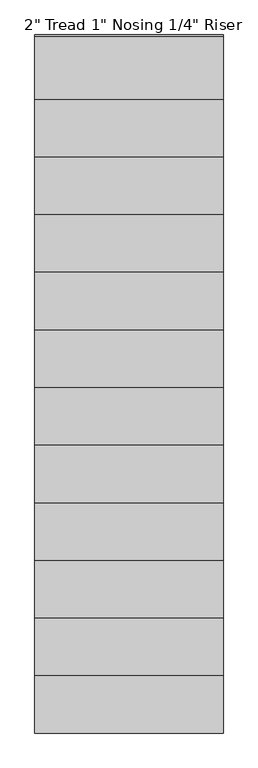
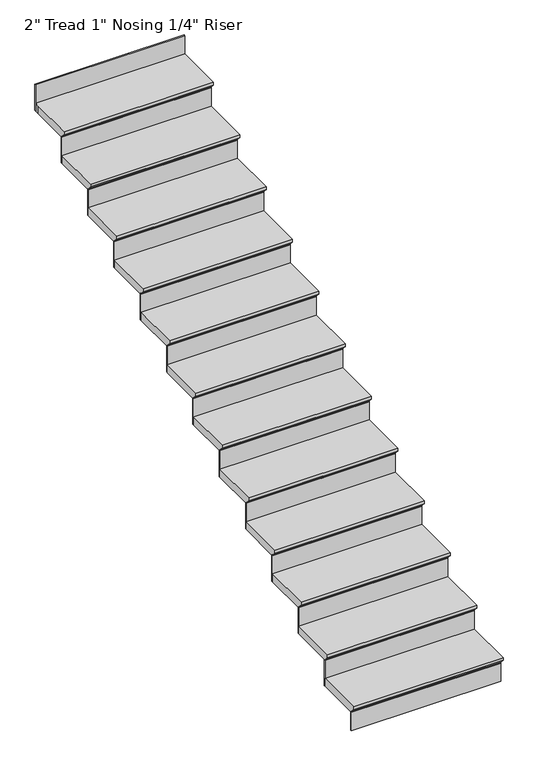
"""IFC4 building model written with IfcOpenShell, lengths in millimetres: stair flight geometry."""

from ifc_helpers import new_model, si_unit, origin, place, context, project, spatial, faceted_brep, source, transform, mapped, element, save


def stair_flight_0d59740e(model_context):
    return source(origin(), model_context, "Body", "Brep", [
        faceted_brep([(-2703.0415084, 19841.9216096, 31480.9005799), (-2703.0415084, 19841.9216096, 31499.9505799), (-3617.4415084, 19841.9216096, 31499.9505799), (-3617.4415084, 19841.9216096, 31480.9005799), (-2703.0415084, 19867.3216096, 31455.5005799), (-3617.4415084, 19867.3216096, 31455.5005799), (-2703.0415084, 20146.7216096, 31499.9505799), (-3617.4415084, 20146.7216096, 31499.9505799), (-3617.4415084, 19867.3216096, 31449.1505799), (-3617.4415084, 20146.7216096, 31449.1505799), (-2703.0415084, 20146.7216096, 31449.1505799), (-2703.0415084, 19867.3216096, 31449.1505799)], [[[0, 1, 2, 3]], [[4, 0, 3, 5]], [[2, 1, 6, 7]], [[8, 9, 10, 11]], [[2, 7, 9, 8, 5, 3]], [[8, 11, 4, 5]], [[6, 1, 0, 4, 11, 10]], [[7, 6, 10, 9]]]),
        faceted_brep([(-2703.0415084, 19867.3216096, 31449.1505799), (-2703.0415084, 19867.3216096, 31330.6172466), (-2703.0415084, 19873.6716096, 31330.6172466), (-2703.0415084, 19873.6716096, 31449.1505799), (-3617.4415084, 19867.3216096, 31449.1505799), (-3617.4415084, 19873.6716096, 31449.1505799), (-3617.4415084, 19873.6716096, 31330.6172466), (-3617.4415084, 19867.3216096, 31330.6172466)], [[[0, 1, 2, 3]], [[4, 5, 6, 7]], [[1, 0, 4, 7]], [[2, 1, 7, 6]], [[3, 2, 6, 5]], [[0, 3, 5, 4]]]),
        faceted_brep([(-2703.0415084, 20146.7216096, 31618.4839133), (-2703.0415084, 20146.7216096, 31449.1505799), (-2703.0415084, 20153.0716096, 31449.1505799), (-2703.0415084, 20153.0716096, 31618.4839133), (-3617.4415084, 20146.7216096, 31618.4839133), (-3617.4415084, 20153.0716096, 31618.4839133), (-3617.4415084, 20153.0716096, 31449.1505799), (-3617.4415084, 20146.7216096, 31449.1505799)], [[[0, 1, 2, 3]], [[4, 5, 6, 7]], [[1, 0, 4, 7]], [[2, 1, 7, 6]], [[3, 2, 6, 5]], [[0, 3, 5, 4]]]),
        faceted_brep([(-3617.4415084, 20121.3216096, 31669.2839133), (-2703.0415084, 20121.3216096, 31669.2839133), (-2703.0415084, 20426.1216096, 31669.2839133), (-3617.4415084, 20426.1216096, 31669.2839133), (-3617.4415084, 20146.7216096, 31618.4839133), (-3617.4415084, 20426.1216096, 31618.4839133), (-2703.0415084, 20426.1216096, 31618.4839133), (-2703.0415084, 20146.7216096, 31618.4839133), (-3617.4415084, 20146.7216096, 31624.8339133), (-3617.4415084, 20121.3216096, 31650.2339133), (-2703.0415084, 20146.7216096, 31624.8339133), (-2703.0415084, 20121.3216096, 31650.2339133)], [[[0, 1, 2, 3]], [[4, 5, 6, 7]], [[0, 3, 5, 4, 8, 9]], [[4, 7, 10, 8]], [[2, 1, 11, 10, 7, 6]], [[3, 2, 6, 5]], [[11, 1, 0, 9]], [[10, 11, 9, 8]]]),
        faceted_brep([(-2703.0415084, 20426.1216096, 31787.8172466), (-2703.0415084, 20426.1216096, 31618.4839133), (-2703.0415084, 20432.4716096, 31618.4839133), (-2703.0415084, 20432.4716096, 31787.8172466), (-3617.4415084, 20426.1216096, 31787.8172466), (-3617.4415084, 20432.4716096, 31787.8172466), (-3617.4415084, 20432.4716096, 31618.4839133), (-3617.4415084, 20426.1216096, 31618.4839133)], [[[0, 1, 2, 3]], [[4, 5, 6, 7]], [[1, 0, 4, 7]], [[2, 1, 7, 6]], [[3, 2, 6, 5]], [[0, 3, 5, 4]]]),
        faceted_brep([(-3617.4415084, 20400.7216096, 31838.6172466), (-2703.0415084, 20400.7216096, 31838.6172466), (-2703.0415084, 20705.5216096, 31838.6172466), (-3617.4415084, 20705.5216096, 31838.6172466), (-3617.4415084, 20426.1216096, 31787.8172466), (-3617.4415084, 20705.5216096, 31787.8172466), (-2703.0415084, 20705.5216096, 31787.8172466), (-2703.0415084, 20426.1216096, 31787.8172466), (-3617.4415084, 20426.1216096, 31794.1672466), (-3617.4415084, 20400.7216096, 31819.5672466), (-2703.0415084, 20426.1216096, 31794.1672466), (-2703.0415084, 20400.7216096, 31819.5672466)], [[[0, 1, 2, 3]], [[4, 5, 6, 7]], [[0, 3, 5, 4, 8, 9]], [[4, 7, 10, 8]], [[2, 1, 11, 10, 7, 6]], [[3, 2, 6, 5]], [[11, 1, 0, 9]], [[10, 11, 9, 8]]]),
        faceted_brep([(-2703.0415084, 20705.5216096, 31957.1505799), (-2703.0415084, 20705.5216096, 31787.8172466), (-2703.0415084, 20711.8716096, 31787.8172466), (-2703.0415084, 20711.8716096, 31957.1505799), (-3617.4415084, 20705.5216096, 31957.1505799), (-3617.4415084, 20711.8716096, 31957.1505799), (-3617.4415084, 20711.8716096, 31787.8172466), (-3617.4415084, 20705.5216096, 31787.8172466)], [[[0, 1, 2, 3]], [[4, 5, 6, 7]], [[1, 0, 4, 7]], [[2, 1, 7, 6]], [[3, 2, 6, 5]], [[0, 3, 5, 4]]]),
        faceted_brep([(-3617.4415084, 20680.1216096, 32007.9505799), (-2703.0415084, 20680.1216096, 32007.9505799), (-2703.0415084, 20984.9216096, 32007.9505799), (-3617.4415084, 20984.9216096, 32007.9505799), (-3617.4415084, 20705.5216096, 31957.1505799), (-3617.4415084, 20984.9216096, 31957.1505799), (-2703.0415084, 20984.9216096, 31957.1505799), (-2703.0415084, 20705.5216096, 31957.1505799), (-3617.4415084, 20705.5216096, 31963.5005799), (-3617.4415084, 20680.1216096, 31988.9005799), (-2703.0415084, 20705.5216096, 31963.5005799), (-2703.0415084, 20680.1216096, 31988.9005799)], [[[0, 1, 2, 3]], [[4, 5, 6, 7]], [[0, 3, 5, 4, 8, 9]], [[4, 7, 10, 8]], [[2, 1, 11, 10, 7, 6]], [[3, 2, 6, 5]], [[11, 1, 0, 9]], [[10, 11, 9, 8]]]),
        faceted_brep([(-2703.0415084, 20984.9216096, 32126.4839133), (-2703.0415084, 20984.9216096, 31957.1505799), (-2703.0415084, 20991.2716096, 31957.1505799), (-2703.0415084, 20991.2716096, 32126.4839133), (-3617.4415084, 20984.9216096, 32126.4839133), (-3617.4415084, 20991.2716096, 32126.4839133), (-3617.4415084, 20991.2716096, 31957.1505799), (-3617.4415084, 20984.9216096, 31957.1505799)], [[[0, 1, 2, 3]], [[4, 5, 6, 7]], [[1, 0, 4, 7]], [[2, 1, 7, 6]], [[3, 2, 6, 5]], [[0, 3, 5, 4]]]),
        faceted_brep([(-3617.4415084, 20959.5216096, 32177.2839133), (-2703.0415084, 20959.5216096, 32177.2839133), (-2703.0415084, 21264.3216096, 32177.2839133), (-3617.4415084, 21264.3216096, 32177.2839133), (-3617.4415084, 20984.9216096, 32126.4839133), (-3617.4415084, 21264.3216096, 32126.4839133), (-2703.0415084, 21264.3216096, 32126.4839133), (-2703.0415084, 20984.9216096, 32126.4839133), (-3617.4415084, 20984.9216096, 32132.8339133), (-3617.4415084, 20959.5216096, 32158.2339133), (-2703.0415084, 20984.9216096, 32132.8339133), (-2703.0415084, 20959.5216096, 32158.2339133)], [[[0, 1, 2, 3]], [[4, 5, 6, 7]], [[0, 3, 5, 4, 8, 9]], [[4, 7, 10, 8]], [[2, 1, 11, 10, 7, 6]], [[3, 2, 6, 5]], [[11, 1, 0, 9]], [[10, 11, 9, 8]]]),
        faceted_brep([(-2703.0415084, 21264.3216096, 32295.8172466), (-2703.0415084, 21264.3216096, 32126.4839133), (-2703.0415084, 21270.6716096, 32126.4839133), (-2703.0415084, 21270.6716096, 32295.8172466), (-3617.4415084, 21264.3216096, 32295.8172466), (-3617.4415084, 21270.6716096, 32295.8172466), (-3617.4415084, 21270.6716096, 32126.4839133), (-3617.4415084, 21264.3216096, 32126.4839133)], [[[0, 1, 2, 3]], [[4, 5, 6, 7]], [[1, 0, 4, 7]], [[2, 1, 7, 6]], [[3, 2, 6, 5]], [[0, 3, 5, 4]]]),
        faceted_brep([(-3617.4415084, 21238.9216096, 32346.6172466), (-2703.0415084, 21238.9216096, 32346.6172466), (-2703.0415084, 21543.7216096, 32346.6172466), (-3617.4415084, 21543.7216096, 32346.6172466), (-3617.4415084, 21264.3216096, 32295.8172466), (-3617.4415084, 21543.7216096, 32295.8172466), (-2703.0415084, 21543.7216096, 32295.8172466), (-2703.0415084, 21264.3216096, 32295.8172466), (-3617.4415084, 21264.3216096, 32302.1672466), (-3617.4415084, 21238.9216096, 32327.5672466), (-2703.0415084, 21264.3216096, 32302.1672466), (-2703.0415084, 21238.9216096, 32327.5672466)], [[[0, 1, 2, 3]], [[4, 5, 6, 7]], [[0, 3, 5, 4, 8, 9]], [[4, 7, 10, 8]], [[2, 1, 11, 10, 7, 6]], [[3, 2, 6, 5]], [[11, 1, 0, 9]], [[10, 11, 9, 8]]]),
        faceted_brep([(-2703.0415084, 21543.7216096, 32465.1505799), (-2703.0415084, 21543.7216096, 32295.8172466), (-2703.0415084, 21550.0716096, 32295.8172466), (-2703.0415084, 21550.0716096, 32465.1505799), (-3617.4415084, 21543.7216096, 32465.1505799), (-3617.4415084, 21550.0716096, 32465.1505799), (-3617.4415084, 21550.0716096, 32295.8172466), (-3617.4415084, 21543.7216096, 32295.8172466)], [[[0, 1, 2, 3]], [[4, 5, 6, 7]], [[1, 0, 4, 7]], [[2, 1, 7, 6]], [[3, 2, 6, 5]], [[0, 3, 5, 4]]]),
        faceted_brep([(-3617.4415084, 21518.3216096, 32515.9505799), (-2703.0415084, 21518.3216096, 32515.9505799), (-2703.0415084, 21823.1216096, 32515.9505799), (-3617.4415084, 21823.1216096, 32515.9505799), (-3617.4415084, 21543.7216096, 32465.1505799), (-3617.4415084, 21823.1216096, 32465.1505799), (-2703.0415084, 21823.1216096, 32465.1505799), (-2703.0415084, 21543.7216096, 32465.1505799), (-3617.4415084, 21543.7216096, 32471.5005799), (-3617.4415084, 21518.3216096, 32496.9005799), (-2703.0415084, 21543.7216096, 32471.5005799), (-2703.0415084, 21518.3216096, 32496.9005799)], [[[0, 1, 2, 3]], [[4, 5, 6, 7]], [[0, 3, 5, 4, 8, 9]], [[4, 7, 10, 8]], [[2, 1, 11, 10, 7, 6]], [[3, 2, 6, 5]], [[11, 1, 0, 9]], [[10, 11, 9, 8]]]),
        faceted_brep([(-2703.0415084, 21823.1216096, 32634.4839133), (-2703.0415084, 21823.1216096, 32465.1505799), (-2703.0415084, 21829.4716096, 32465.1505799), (-2703.0415084, 21829.4716096, 32634.4839133), (-3617.4415084, 21823.1216096, 32634.4839133), (-3617.4415084, 21829.4716096, 32634.4839133), (-3617.4415084, 21829.4716096, 32465.1505799), (-3617.4415084, 21823.1216096, 32465.1505799)], [[[0, 1, 2, 3]], [[4, 5, 6, 7]], [[1, 0, 4, 7]], [[2, 1, 7, 6]], [[3, 2, 6, 5]], [[0, 3, 5, 4]]]),
        faceted_brep([(-3617.4415084, 21797.7216096, 32685.2839133), (-2703.0415084, 21797.7216096, 32685.2839133), (-2703.0415084, 22102.5216096, 32685.2839133), (-3617.4415084, 22102.5216096, 32685.2839133), (-3617.4415084, 21823.1216096, 32634.4839133), (-3617.4415084, 22102.5216096, 32634.4839133), (-2703.0415084, 22102.5216096, 32634.4839133), (-2703.0415084, 21823.1216096, 32634.4839133), (-3617.4415084, 21823.1216096, 32640.8339133), (-3617.4415084, 21797.7216096, 32666.2339133), (-2703.0415084, 21823.1216096, 32640.8339133), (-2703.0415084, 21797.7216096, 32666.2339133)], [[[0, 1, 2, 3]], [[4, 5, 6, 7]], [[0, 3, 5, 4, 8, 9]], [[4, 7, 10, 8]], [[2, 1, 11, 10, 7, 6]], [[3, 2, 6, 5]], [[11, 1, 0, 9]], [[10, 11, 9, 8]]]),
        faceted_brep([(-2703.0415084, 22102.5216096, 32803.8172466), (-2703.0415084, 22102.5216096, 32634.4839133), (-2703.0415084, 22108.8716096, 32634.4839133), (-2703.0415084, 22108.8716096, 32803.8172466), (-3617.4415084, 22102.5216096, 32803.8172466), (-3617.4415084, 22108.8716096, 32803.8172466), (-3617.4415084, 22108.8716096, 32634.4839133), (-3617.4415084, 22102.5216096, 32634.4839133)], [[[0, 1, 2, 3]], [[4, 5, 6, 7]], [[1, 0, 4, 7]], [[2, 1, 7, 6]], [[3, 2, 6, 5]], [[0, 3, 5, 4]]]),
        faceted_brep([(-3617.4415084, 22077.1216096, 32854.6172466), (-2703.0415084, 22077.1216096, 32854.6172466), (-2703.0415084, 22381.9216096, 32854.6172466), (-3617.4415084, 22381.9216096, 32854.6172466), (-3617.4415084, 22102.5216096, 32803.8172466), (-3617.4415084, 22381.9216096, 32803.8172466), (-2703.0415084, 22381.9216096, 32803.8172466), (-2703.0415084, 22102.5216096, 32803.8172466), (-3617.4415084, 22102.5216096, 32810.1672466), (-3617.4415084, 22077.1216096, 32835.5672466), (-2703.0415084, 22102.5216096, 32810.1672466), (-2703.0415084, 22077.1216096, 32835.5672466)], [[[0, 1, 2, 3]], [[4, 5, 6, 7]], [[0, 3, 5, 4, 8, 9]], [[4, 7, 10, 8]], [[2, 1, 11, 10, 7, 6]], [[3, 2, 6, 5]], [[11, 1, 0, 9]], [[10, 11, 9, 8]]]),
        faceted_brep([(-2703.0415084, 22381.9216096, 32973.1505799), (-2703.0415084, 22381.9216096, 32803.8172466), (-2703.0415084, 22388.2716096, 32803.8172466), (-2703.0415084, 22388.2716096, 32973.1505799), (-3617.4415084, 22381.9216096, 32973.1505799), (-3617.4415084, 22388.2716096, 32973.1505799), (-3617.4415084, 22388.2716096, 32803.8172466), (-3617.4415084, 22381.9216096, 32803.8172466)], [[[0, 1, 2, 3]], [[4, 5, 6, 7]], [[1, 0, 4, 7]], [[2, 1, 7, 6]], [[3, 2, 6, 5]], [[0, 3, 5, 4]]]),
        faceted_brep([(-3617.4415084, 22356.5216096, 33023.9505799), (-2703.0415084, 22356.5216096, 33023.9505799), (-2703.0415084, 22661.3216096, 33023.9505799), (-3617.4415084, 22661.3216096, 33023.9505799), (-3617.4415084, 22381.9216096, 32973.1505799), (-3617.4415084, 22661.3216096, 32973.1505799), (-2703.0415084, 22661.3216096, 32973.1505799), (-2703.0415084, 22381.9216096, 32973.1505799), (-3617.4415084, 22381.9216096, 32979.5005799), (-3617.4415084, 22356.5216096, 33004.9005799), (-2703.0415084, 22381.9216096, 32979.5005799), (-2703.0415084, 22356.5216096, 33004.9005799)], [[[0, 1, 2, 3]], [[4, 5, 6, 7]], [[0, 3, 5, 4, 8, 9]], [[4, 7, 10, 8]], [[2, 1, 11, 10, 7, 6]], [[3, 2, 6, 5]], [[11, 1, 0, 9]], [[10, 11, 9, 8]]]),
        faceted_brep([(-2703.0415084, 22661.3216096, 33142.4839133), (-2703.0415084, 22661.3216096, 32973.1505799), (-2703.0415084, 22667.6716096, 32973.1505799), (-2703.0415084, 22667.6716096, 33142.4839133), (-3617.4415084, 22661.3216096, 33142.4839133), (-3617.4415084, 22667.6716096, 33142.4839133), (-3617.4415084, 22667.6716096, 32973.1505799), (-3617.4415084, 22661.3216096, 32973.1505799)], [[[0, 1, 2, 3]], [[4, 5, 6, 7]], [[1, 0, 4, 7]], [[2, 1, 7, 6]], [[3, 2, 6, 5]], [[0, 3, 5, 4]]]),
        faceted_brep([(-3617.4415084, 22635.9216096, 33193.2839133), (-2703.0415084, 22635.9216096, 33193.2839133), (-2703.0415084, 22940.7216096, 33193.2839133), (-3617.4415084, 22940.7216096, 33193.2839133), (-3617.4415084, 22661.3216096, 33142.4839133), (-3617.4415084, 22940.7216096, 33142.4839133), (-2703.0415084, 22940.7216096, 33142.4839133), (-2703.0415084, 22661.3216096, 33142.4839133), (-3617.4415084, 22661.3216096, 33148.8339133), (-3617.4415084, 22635.9216096, 33174.2339133), (-2703.0415084, 22661.3216096, 33148.8339133), (-2703.0415084, 22635.9216096, 33174.2339133)], [[[0, 1, 2, 3]], [[4, 5, 6, 7]], [[0, 3, 5, 4, 8, 9]], [[4, 7, 10, 8]], [[2, 1, 11, 10, 7, 6]], [[3, 2, 6, 5]], [[11, 1, 0, 9]], [[10, 11, 9, 8]]]),
        faceted_brep([(-2703.0415084, 23220.1216096, 33481.1505799), (-2703.0415084, 23220.1216096, 33311.8172466), (-2703.0415084, 23226.4716096, 33311.8172466), (-2703.0415084, 23226.4716096, 33481.1505799), (-3617.4415084, 23220.1216096, 33481.1505799), (-3617.4415084, 23226.4716096, 33481.1505799), (-3617.4415084, 23226.4716096, 33311.8172466), (-3617.4415084, 23220.1216096, 33311.8172466)], [[[0, 1, 2, 3]], [[4, 5, 6, 7]], [[1, 0, 4, 7]], [[2, 1, 7, 6]], [[3, 2, 6, 5]], [[0, 3, 5, 4]]]),
        faceted_brep([(-2703.0415084, 22940.7216096, 33311.8172466), (-2703.0415084, 22940.7216096, 33142.4839133), (-2703.0415084, 22947.0716096, 33142.4839133), (-2703.0415084, 22947.0716096, 33311.8172466), (-3617.4415084, 22940.7216096, 33311.8172466), (-3617.4415084, 22947.0716096, 33311.8172466), (-3617.4415084, 22947.0716096, 33142.4839133), (-3617.4415084, 22940.7216096, 33142.4839133)], [[[0, 1, 2, 3]], [[4, 5, 6, 7]], [[1, 0, 4, 7]], [[2, 1, 7, 6]], [[3, 2, 6, 5]], [[0, 3, 5, 4]]]),
        faceted_brep([(-3617.4415084, 23220.1216096, 33362.6172466), (-3617.4415084, 23194.7216096, 33362.6172466), (-3617.4415084, 22915.3216096, 33362.6172466), (-2703.0415084, 22915.3216096, 33362.6172466), (-2703.0415084, 23220.1216096, 33362.6172466), (-3617.4415084, 23194.7216096, 33311.8172466), (-3617.4415084, 23220.1216096, 33311.8172466), (-2703.0415084, 23220.1216096, 33311.8172466), (-2703.0415084, 22940.7216096, 33311.8172466), (-3617.4415084, 22940.7216096, 33311.8172466), (-3617.4415084, 22940.7216096, 33318.1672466), (-3617.4415084, 22915.3216096, 33343.5672466), (-2703.0415084, 22940.7216096, 33318.1672466), (-2703.0415084, 22915.3216096, 33343.5672466)], [[[0, 1, 2, 3, 4]], [[5, 6, 7, 8, 9]], [[1, 0, 6, 5]], [[2, 1, 5, 9, 10, 11]], [[9, 8, 12, 10]], [[4, 3, 13, 12, 8, 7]], [[0, 4, 7, 6]], [[13, 3, 2, 11]], [[12, 13, 11, 10]]]),
    ])


if __name__ == "__main__":
    model = new_model("IFC4")
    model_context = context("Model", 3, world=origin())
    ifc_project = project(units=[si_unit("LENGTHUNIT", "METRE", prefix="MILLI")], contexts=[model_context])
    site = spatial("IfcSite", under=ifc_project)
    building = spatial("IfcBuilding", under=site)
    placement = place(None, origin())
    stair_flight_shape = stair_flight_0d59740e(model_context)
    element("IfcStairFlight", 1, ObjectType="2\" Tread 1\" Nosing 1/4\" Riser", at=placement, inside=building, context=model_context, shape_type="MappedRepresentation", body=[
        mapped(stair_flight_shape, transform((0.0, 0.0, 0.0), x_axis=(1.0, 0.0, 0.0), y_axis=(0.0, 1.0, 0.0), z_axis=(0.0, 0.0, 1.0))),
    ])
    save(model, "model.ifc")
